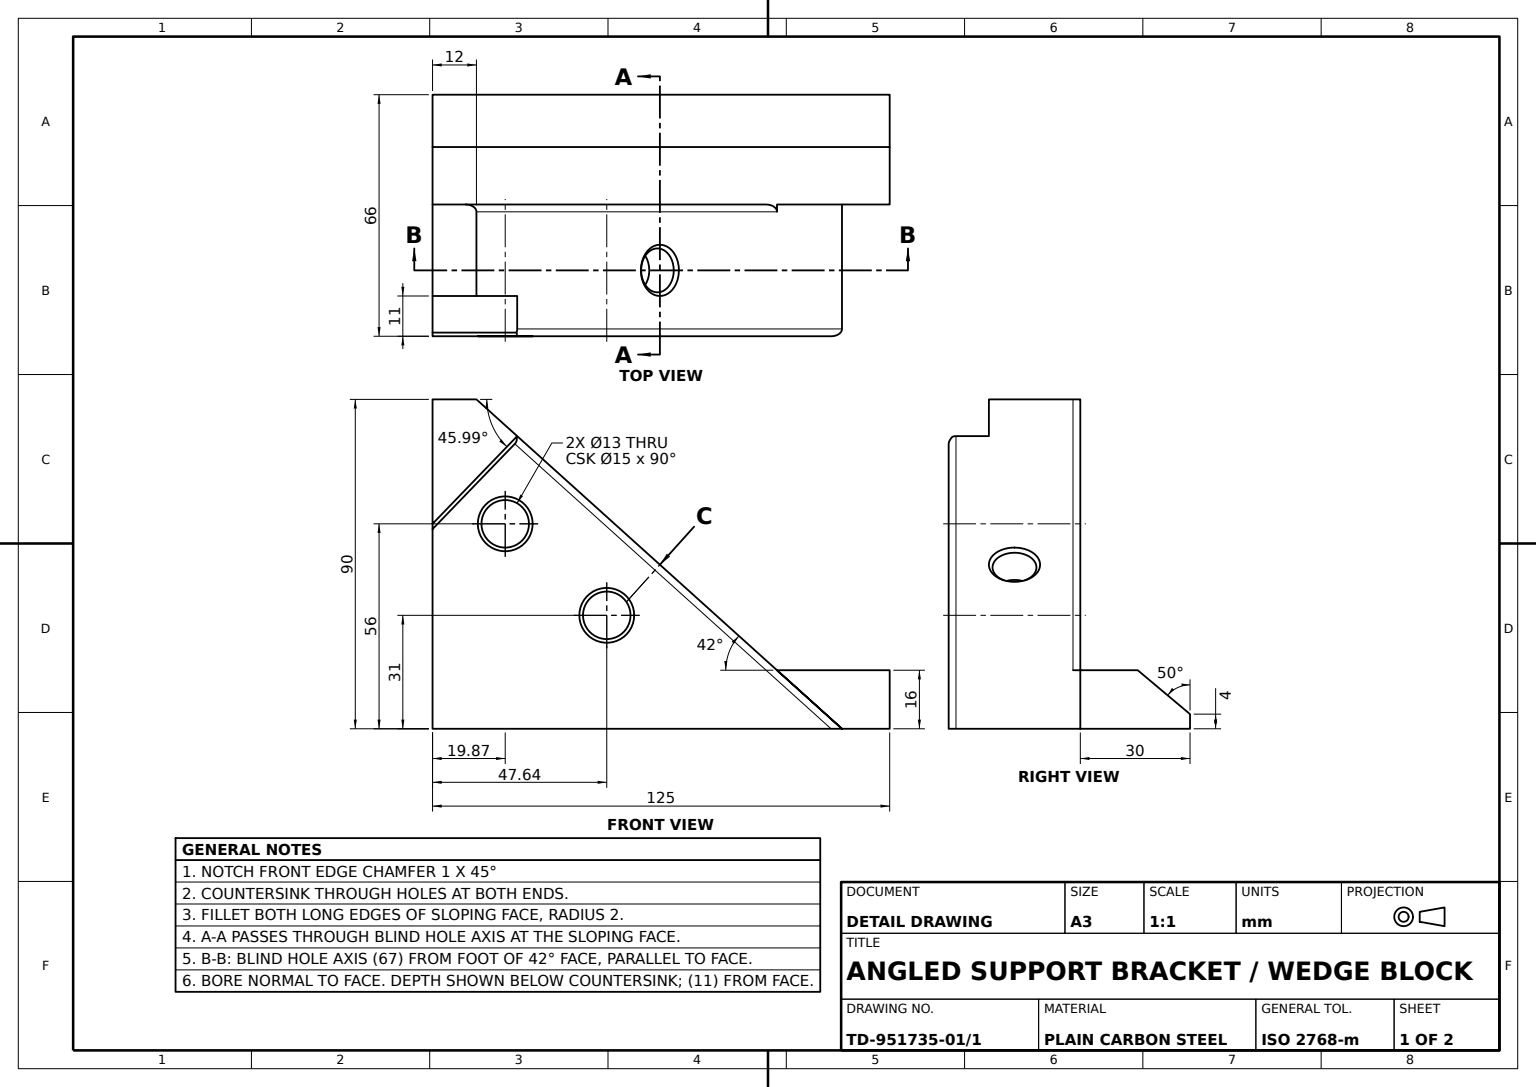
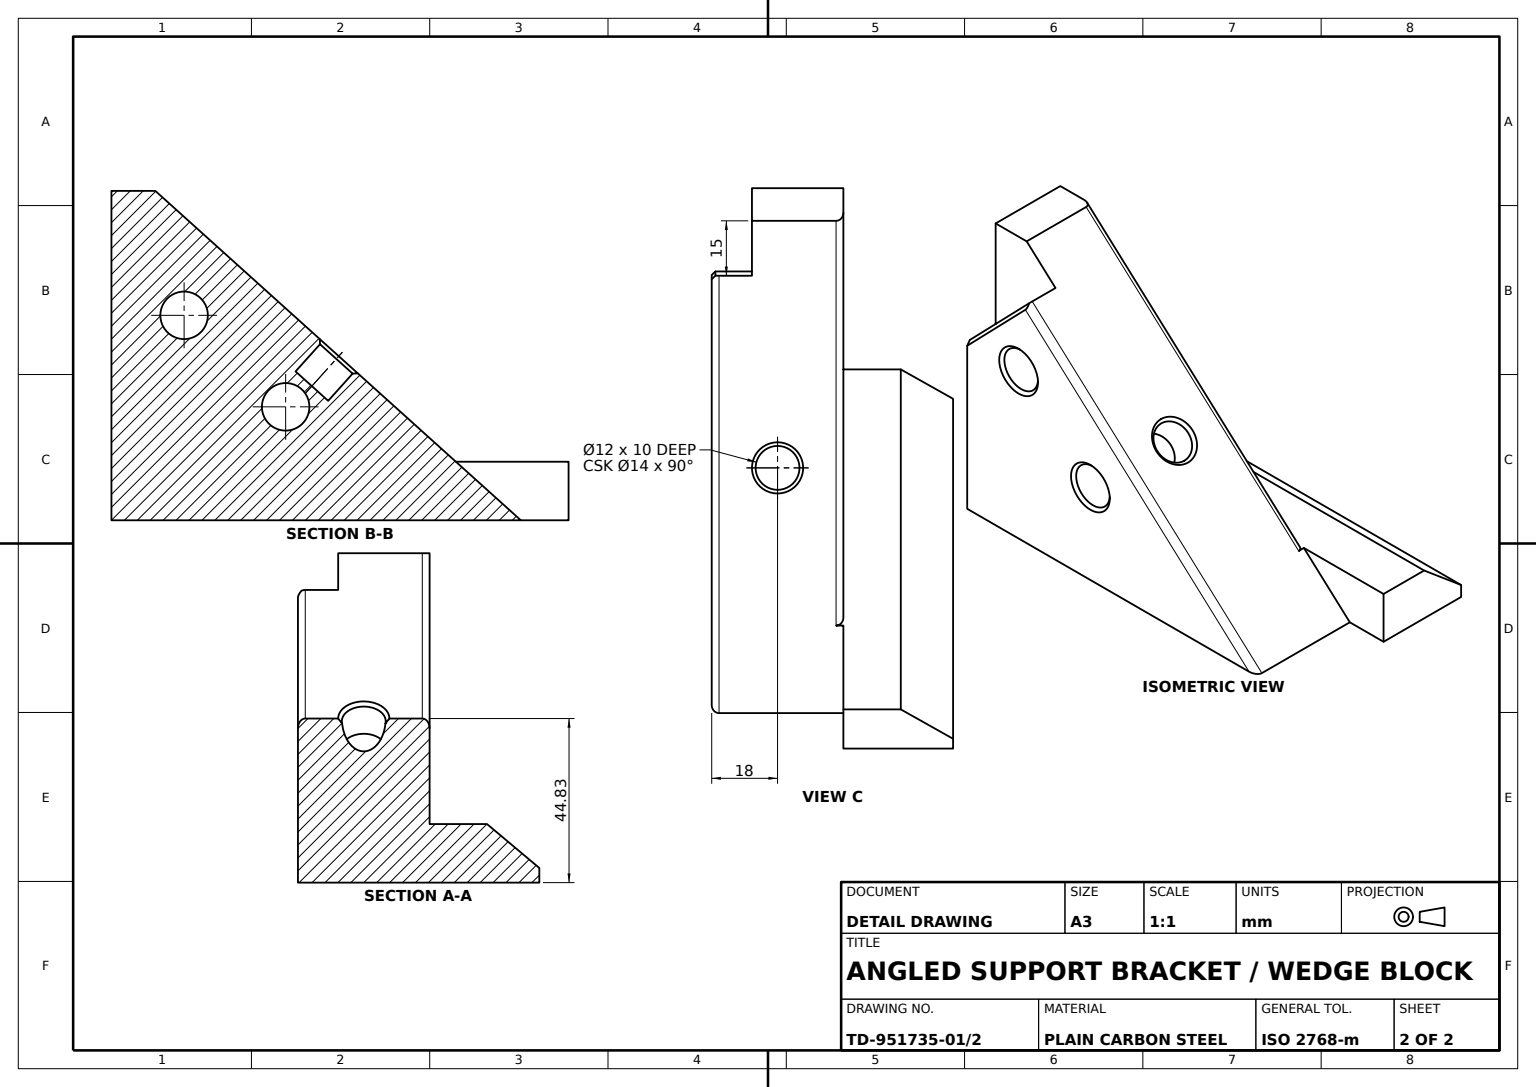
from build123d import *

# Parameters (mm, degrees)
TRIANGULAR_BRACKET_BODY_DEPTH    = 18
RECTANGULAR_CUT_15X56_DEPTH      = 11
HOLE_SKETCH_R                    = 6
HOLE_CUT_DEPTH                   = 11
SLIDE_RAIL_125_DEPTH             = 125
RAIL_GROOVE_SKETCH_R             = 6.5
RAIL_GROOVE_CUT_DEPTH            = 125
RECTANGULAR_CUT_CHAMFER_1MM_SIZE = 1
HOLE_AND_GROOVE_CHAMFER_1MM_SIZE = 1
BODY_EDGE_FILLET_R2_A_R          = 2
BODY_EDGE_FILLET_R2_B_R          = 2


with BuildPart() as part:
    # Bracket Profile Sketch → Triangular Bracket Body (new, symmetric)
    with BuildSketch(Plane.XY):
        Polygon((0, 0), (111.955126335, 0), (12, 90), (0, 90), align=None)
    extrude(amount=TRIANGULAR_BRACKET_BODY_DEPTH, both=True)

    # Rectangular Cut Sketch → Rectangular Cut 15x56 (cut)
    with BuildSketch(Plane.XY.offset(18)):
        Polygon((23.147172382, 79.963040905), (0, 56), (0, 90), (12, 90), align=None)
    extrude(amount=-RECTANGULAR_CUT_15X56_DEPTH, mode=Mode.SUBTRACT)

    # Hole Sketch → Hole Cut (cut)
    with BuildSketch(Plane(origin=(50.126314512, 55.670912219, 0), x_dir=(0.743144825477398, -0.669130606358854, 0), z_dir=(0.669130606358854, 0.743144825477398, 0))):
        with Locations(Location((16.198872821, 0, 0), (0, 0, 180))):
            Circle(HOLE_SKETCH_R)
    extrude(amount=-HOLE_CUT_DEPTH, mode=Mode.SUBTRACT)

    # Slide Rail Profile Sketch → Slide Rail 125 (add)
    with BuildSketch(Plane.ZY):
        Polygon((-18, 16), (-33.698956889, 16), (-48, 4), (-48, 0), (-18, 0), align=None)
    extrude(amount=-SLIDE_RAIL_125_DEPTH)

    # Rail Groove Sketch → Rail Groove Cut (cut)
    with BuildSketch(Plane(origin=(0, 0, -18), x_dir=(-1, 0, 0), z_dir=(0, 0, -1))):
        with Locations((-47.636607378, 31)):
            Circle(RAIL_GROOVE_SKETCH_R)
        with Locations((-19.871294507, 56)):
            Circle(RAIL_GROOVE_SKETCH_R)
    extrude(amount=-RAIL_GROOVE_CUT_DEPTH, mode=Mode.SUBTRACT)

    # Rectangular Cut Chamfer 1mm
    rectangular_cut_chamfer_1mm_edges = [part.edges().sort_by_distance(p)[0] for p in [
        (11.573586191, 67.981520452, 18),
    ]]
    chamfer(rectangular_cut_chamfer_1mm_edges, length=RECTANGULAR_CUT_CHAMFER_1MM_SIZE)

    # Hole and Groove Chamfer 1mm
    hole_and_groove_chamfer_1mm_edges = [part.edges().sort_by_distance(p)[0] for p in [
        (66.623291981, 40.816966988, 0),
        (54.136607378, 31, 18),
        (54.136607378, 31, -18),
        (26.371294507, 56, 18),
        (26.371294507, 56, -18),
    ]]
    chamfer(hole_and_groove_chamfer_1mm_edges, length=HOLE_AND_GROOVE_CHAMFER_1MM_SIZE)

    # Body Edge Fillet R2 A
    body_edge_fillet_r2_a_edges = [part.edges().sort_by_distance(p)[0] for p in [
        (53.092663049, 53, -18),
    ]]
    fillet(body_edge_fillet_r2_a_edges, radius=BODY_EDGE_FILLET_R2_A_R)

    # Body Edge Fillet R2 B
    body_edge_fillet_r2_b_edges = [part.edges().sort_by_distance(p)[0] for p in [
        (67.92295004, 39.646749615, 18),
    ]]
    fillet(body_edge_fillet_r2_b_edges, radius=BODY_EDGE_FILLET_R2_B_R)


solid = part.part
